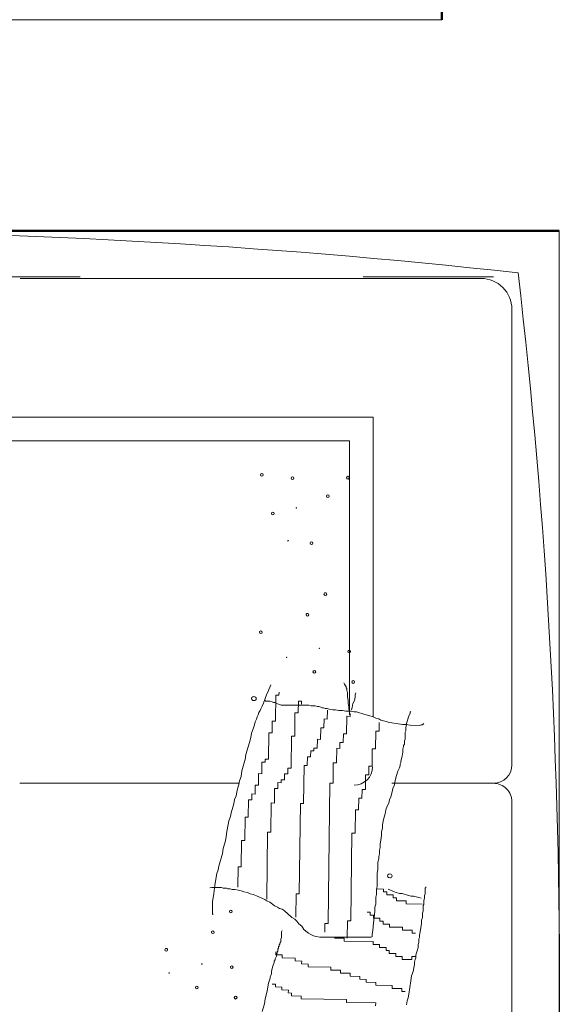
# Model space of a CAD drawing. Units: inches. Extents: x -466983 to 1020, y 324 to 318697.
# Tile 91 of 97: x 787 to 810, y 921 to 963. Entities that reach past the tile are written whole.
import ezdxf

# ---------------------------------------------------------------- set-up
doc = ezdxf.new("R2010")
doc.units = ezdxf.units.IN
doc.header["$MEASUREMENT"] = 0
for name, color, linetype, lineweight in [('A-FLOR-PATT', 252, 'Continuous', 13), ('A-FURN', 8, 'Continuous', 18), ('A-WALL', 7, 'Continuous', 50), ('L-SITE', 3, 'Continuous', 18)]:
    doc.layers.add(name, color=color, linetype=linetype, lineweight=lineweight)

# ---------------------------------------------------------------- blocks, each defined once
blk = doc.blocks.new('L Shaped Sofa')
at = {"ltscale": 2}
for p, q in [((2475.263, 723.229), (2475.263, 821.686)), ((2458.96, 739.532), (2458.96, 802.773)), ((2460.8, 737.692), (2460.8, 802.773)), ((2471.701, 760.482), (2471.701, 766.134)), ((2432.347, 748.121), (2432.347, 765.179)), ((2471.575, 729.305), (2471.575, 765.138)), ((2422.162, 750.193), (2423.138, 750.189)), ((2422.21, 750.139), (2422.162, 750.193)), ((2423.138, 750.189), (2423.772, 750.077)), ((2423.772, 750.077), (2424.406, 750.02)), ((2424.26, 750.238), (2424.213, 750.4)), ((2424.256, 749.479), (2424.26, 750.238)), ((2424.406, 750.02), (2424.747, 749.964)), ((2424.747, 749.964), (2425.332, 749.853)), ((2425.332, 749.853), (2425.624, 749.743)), ((2424.154, 748.828), (2424.155, 748.991)), ((2424.155, 748.991), (2424.205, 749.099)), ((2424.205, 749.099), (2424.206, 749.37)), ((2424.206, 749.37), (2424.256, 749.479)), ((2425.624, 749.743), (2425.916, 749.688)), ((2425.916, 749.688), (2426.89, 749.412)), ((2426.89, 749.412), (2427.28, 749.356)), ((2427.28, 749.356), (2427.865, 749.191)), ((2427.865, 749.191), (2428.206, 749.135)), ((2428.206, 749.135), (2428.596, 749.079)), ((2428.596, 749.079), (2429.132, 748.968)), ((2424.053, 748.178), (2424.103, 748.449)), ((2424.103, 748.449), (2424.104, 748.666)), ((2424.104, 748.666), (2424.154, 748.828)), ((2424.269, 748.227), (2425.857, 748.207)), ((2429.132, 748.968), (2429.425, 748.912)), ((2429.425, 748.912), (2429.766, 748.802)), ((2429.766, 748.802), (2430.058, 748.747)), ((2430.058, 748.747), (2430.74, 748.526)), ((2430.74, 748.526), (2431.081, 748.471)), ((2431.081, 748.471), (2431.373, 748.361)), ((2431.373, 748.361), (2431.666, 748.305)), ((2431.666, 748.305), (2431.909, 748.25)), ((2431.909, 748.25), (2432.25, 748.14)), ((2423.754, 747.258), (2423.853, 747.474)), ((2423.853, 747.474), (2423.904, 747.745)), ((2423.904, 747.745), (2424.003, 747.962)), ((2424.003, 747.962), (2424.053, 748.178)), ((2425.857, 748.207), (2425.853, 747.956)), ((2425.853, 747.956), (2427.895, 747.931)), ((2427.895, 747.931), (2427.892, 747.679)), ((2427.892, 747.679), (2429.707, 747.657)), ((2429.707, 747.657), (2429.704, 747.405)), ((2432.25, 748.14), (2432.543, 748.084)), ((2432.543, 748.084), (2432.884, 747.974)), ((2432.884, 747.974), (2433.322, 747.918)), ((2433.322, 747.918), (2433.858, 747.753)), ((2433.858, 747.753), (2434.199, 747.643)), ((2434.199, 747.643), (2434.589, 747.587)), ((2434.589, 747.587), (2435.174, 747.421)), ((2423.308, 746.122), (2423.605, 746.771)), ((2423.605, 746.771), (2423.704, 747.041)), ((2423.704, 747.041), (2423.754, 747.258)), ((2429.704, 747.405), (2431.065, 747.388)), ((2431.065, 747.388), (2431.061, 747.136)), ((2431.061, 747.136), (2431.515, 747.131)), ((2431.515, 747.131), (2431.512, 746.879)), ((2431.512, 746.879), (2432.193, 746.87)), ((2432.193, 746.87), (2432.19, 746.618)), ((2435.174, 747.421), (2435.515, 747.311)), ((2435.515, 747.311), (2435.904, 747.201)), ((2435.904, 747.201), (2436.246, 747.145)), ((2436.246, 747.145), (2436.586, 747.035)), ((2436.586, 747.035), (2436.879, 746.925)), ((2436.879, 746.925), (2437.122, 746.87)), ((2437.122, 746.87), (2437.317, 746.761)), ((2437.317, 746.761), (2437.512, 746.705)), ((2437.512, 746.705), (2437.658, 746.651)), ((2414.624, 746.325), (2415.208, 746.16)), ((2415.208, 746.16), (2415.598, 746.104)), ((2415.598, 746.104), (2416.183, 745.938)), ((2416.183, 745.938), (2416.524, 745.882)), ((2423.111, 745.743), (2423.21, 745.959)), ((2423.21, 745.959), (2423.308, 746.122)), ((2423.334, 745.971), (2428.551, 745.907)), ((2432.19, 746.618), (2433.097, 746.607)), ((2433.097, 746.607), (2433.094, 746.355)), ((2433.094, 746.355), (2434.001, 746.344)), ((2434.001, 746.344), (2433.998, 746.092)), ((2433.998, 746.092), (2434.225, 746.09)), ((2434.225, 746.09), (2434.222, 745.838)), ((2437.658, 746.651), (2437.852, 746.595)), ((2437.852, 746.595), (2437.998, 746.486)), ((2437.998, 746.486), (2438.144, 746.431)), ((2438.144, 746.431), (2438.339, 746.322)), ((2438.339, 746.322), (2438.582, 746.213)), ((2438.582, 746.213), (2438.923, 746.102)), ((2438.725, 745.724), (2438.727, 746.049)), ((2438.727, 746.049), (2438.777, 746.103)), ((2438.923, 746.102), (2439.215, 745.993)), ((2439.215, 745.993), (2439.556, 745.828)), ((2416.513, 744.794), (2416.519, 745.298)), ((2416.519, 745.298), (2416.746, 745.295)), ((2416.524, 745.882), (2416.816, 745.827)), ((2416.746, 745.295), (2416.749, 745.547)), ((2416.816, 745.827), (2417.06, 745.771)), ((2417.06, 745.771), (2417.206, 745.716)), ((2417.206, 745.716), (2417.304, 745.716)), ((2417.304, 745.716), (2417.401, 745.661)), ((2417.401, 745.661), (2417.547, 745.606)), ((2417.547, 745.606), (2417.742, 745.605)), ((2417.742, 745.605), (2418.132, 745.495)), ((2418.132, 745.495), (2418.424, 745.385)), ((2418.424, 745.385), (2418.522, 745.385)), ((2418.522, 745.385), (2418.619, 745.33)), ((2418.619, 745.33), (2418.716, 745.33)), ((2418.716, 745.33), (2418.911, 745.22)), ((2418.911, 745.22), (2419.057, 745.22)), ((2419.008, 744.764), (2419.015, 745.268)), ((2419.015, 745.268), (2419.241, 745.265)), ((2419.057, 745.22), (2419.155, 745.165)), ((2419.155, 745.165), (2419.252, 745.165)), ((2419.252, 745.165), (2419.301, 745.11)), ((2422.717, 745.148), (2422.816, 745.365)), ((2422.816, 745.365), (2422.963, 745.527)), ((2422.963, 745.527), (2423.111, 745.743)), ((2428.551, 745.907), (2428.548, 745.655)), ((2428.548, 745.655), (2430.816, 745.627)), ((2430.816, 745.627), (2430.813, 745.375)), ((2430.813, 745.375), (2431.947, 745.362)), ((2431.947, 745.362), (2431.944, 745.11)), ((2434.222, 745.838), (2436.263, 745.813)), ((2436.263, 745.813), (2436.26, 745.561)), ((2436.26, 745.561), (2437.168, 745.55)), ((2437.168, 745.55), (2437.165, 745.298)), ((2437.165, 745.298), (2439.206, 745.273)), ((2438.527, 745.128), (2438.626, 745.345)), ((2438.626, 745.453), (2438.676, 745.561)), ((2438.626, 745.345), (2438.626, 745.453)), ((2438.676, 745.561), (2438.725, 745.724)), ((2439.206, 745.273), (2439.203, 745.021)), ((2439.556, 745.828), (2439.994, 745.664)), ((2416.28, 744.293), (2416.286, 744.797)), ((2416.286, 744.797), (2416.513, 744.794)), ((2418.769, 743.759), (2418.782, 744.767)), ((2418.782, 744.767), (2419.008, 744.764)), ((2419.301, 745.11), (2419.447, 745.11)), ((2419.447, 745.11), (2419.544, 745.055)), ((2419.544, 745.055), (2419.642, 745.054)), ((2419.642, 745.054), (2419.69, 745)), ((2419.69, 745), (2419.788, 744.999)), ((2419.788, 744.999), (2419.836, 744.945)), ((2419.836, 744.945), (2419.934, 744.945)), ((2419.934, 744.945), (2420.031, 744.89)), ((2420.031, 744.89), (2420.226, 744.889)), ((2420.226, 744.889), (2420.372, 744.834)), ((2420.372, 744.834), (2420.812, 744.832)), ((2420.812, 744.832), (2420.909, 744.777)), ((2421.929, 744.014), (2422.469, 744.607)), ((2422.469, 744.607), (2422.568, 744.77)), ((2422.568, 744.77), (2422.618, 744.986)), ((2422.618, 744.986), (2422.717, 745.148)), ((2431.944, 745.11), (2432.398, 745.104)), ((2432.398, 745.104), (2432.395, 744.852)), ((2432.395, 744.852), (2432.622, 744.849)), ((2432.622, 744.849), (2432.619, 744.598)), ((2432.619, 744.598), (2433.072, 744.592)), ((2433.072, 744.592), (2433.069, 744.34)), ((2438.414, 742.689), (2438.427, 744.858)), ((2438.427, 744.858), (2438.477, 744.966)), ((2438.477, 744.966), (2438.527, 745.128)), ((2439.43, 745.018), (2439.203, 745.021)), ((2439.203, 745.021), (2439.43, 745.018)), ((2415.814, 743.291), (2415.823, 744.047)), ((2415.823, 744.047), (2416.05, 744.044)), ((2416.05, 744.044), (2416.053, 744.296)), ((2416.053, 744.296), (2416.28, 744.293)), ((2418.536, 743.258), (2418.542, 743.762)), ((2418.542, 743.762), (2418.769, 743.759)), ((2421.438, 743.474), (2421.634, 743.635)), ((2421.634, 743.635), (2421.781, 743.797)), ((2421.781, 743.797), (2421.929, 744.014)), ((2421.945, 743.72), (2423.76, 743.698)), ((2423.76, 743.698), (2423.757, 743.446)), ((2433.069, 744.34), (2433.523, 744.335)), ((2433.523, 744.335), (2433.52, 744.083)), ((2433.52, 744.083), (2436.015, 744.052)), ((2436.015, 744.052), (2436.012, 743.8)), ((2436.012, 743.8), (2437.827, 743.778)), ((2437.827, 743.778), (2437.823, 743.526)), ((2415.544, 739.767), (2415.587, 743.294)), ((2415.587, 743.294), (2415.814, 743.291)), ((2418.303, 742.757), (2418.309, 743.261)), ((2418.309, 743.261), (2418.536, 743.258)), ((2420.701, 742.718), (2420.849, 742.934)), ((2420.849, 742.934), (2420.996, 743.096)), ((2420.996, 743.096), (2421.241, 743.258)), ((2421.241, 743.258), (2421.438, 743.474)), ((2423.757, 743.446), (2430.788, 743.36)), ((2430.788, 743.36), (2430.785, 743.108)), ((2430.785, 743.108), (2433.734, 743.072)), ((2433.734, 743.072), (2433.731, 742.82)), ((2437.823, 743.526), (2438.731, 743.515)), ((2438.728, 743.263), (2438.501, 743.266)), ((2438.731, 743.515), (2438.728, 743.263)), ((2418.055, 740.996), (2418.076, 742.76)), ((2418.076, 742.76), (2418.303, 742.757)), ((2420.403, 741.852), (2420.453, 742.123)), ((2420.453, 742.123), (2420.504, 742.339)), ((2420.504, 742.339), (2420.603, 742.556)), ((2420.603, 742.556), (2420.701, 742.718)), ((2433.731, 742.82), (2434.412, 742.812)), ((2434.412, 742.812), (2434.409, 742.56)), ((2434.409, 742.56), (2434.862, 742.555)), ((2434.862, 742.555), (2434.859, 742.303)), ((2434.859, 742.303), (2435.086, 742.3)), ((2435.086, 742.3), (2435.083, 742.048)), ((2438.312, 742.039), (2438.362, 742.201)), ((2438.362, 742.201), (2438.364, 742.527)), ((2438.364, 742.527), (2438.414, 742.689)), ((2420.378, 737.84), (2420.403, 741.852)), ((2420.783, 741.467), (2421.464, 741.459)), ((2421.464, 741.459), (2421.46, 741.207)), ((2435.083, 742.048), (2435.764, 742.04)), ((2435.764, 742.04), (2435.76, 741.788)), ((2435.76, 741.788), (2436.668, 741.777)), ((2436.668, 741.777), (2436.665, 741.525)), ((2436.665, 741.525), (2437.345, 741.516)), ((2437.345, 741.516), (2437.342, 741.265)), ((2438.161, 741.281), (2438.162, 741.443)), ((2438.162, 741.443), (2438.212, 741.552)), ((2438.212, 741.552), (2438.213, 741.66)), ((2438.213, 741.66), (2438.262, 741.768)), ((2438.262, 741.768), (2438.312, 741.931)), ((2438.312, 741.931), (2438.312, 742.039)), ((2417.819, 740.243), (2417.828, 740.999)), ((2417.828, 740.999), (2418.055, 740.996)), ((2420.311, 739.961), (2420.32, 740.717)), ((2421.46, 741.207), (2432.349, 741.074)), ((2432.349, 741.074), (2432.346, 740.822)), ((2432.346, 740.822), (2433.933, 740.802)), ((2433.933, 740.802), (2433.93, 740.55)), ((2437.342, 741.265), (2438.023, 741.256)), ((2438.009, 740.36), (2438.06, 740.631)), ((2438.06, 740.631), (2438.061, 740.847)), ((2438.061, 740.847), (2438.112, 741.118)), ((2438.112, 741.118), (2438.161, 741.281)), ((2417.583, 739.49), (2417.592, 740.246)), ((2417.592, 740.246), (2417.819, 740.243)), ((2420.056, 737.696), (2420.084, 739.964)), ((2420.084, 739.964), (2420.311, 739.961)), ((2433.93, 740.55), (2435.065, 740.536)), ((2435.065, 740.536), (2435.061, 740.285)), ((2435.061, 740.285), (2435.515, 740.279)), ((2435.515, 740.279), (2435.512, 740.027)), ((2435.512, 740.027), (2436.193, 740.019)), ((2436.193, 740.019), (2436.189, 739.767)), ((2437.955, 739.384), (2437.957, 739.818)), ((2437.957, 739.818), (2438.008, 740.089)), ((2438.008, 740.089), (2438.009, 740.36)), ((2439.714, 739.755), (2439.763, 739.809)), ((2439.763, 739.809), (2439.86, 739.809)), ((2439.86, 739.809), (2439.909, 739.863)), ((2439.909, 739.863), (2440.056, 739.916)), ((2440.056, 739.916), (2440.154, 739.97)), ((2415.29, 737.503), (2415.317, 739.77)), ((2415.317, 739.77), (2415.544, 739.767)), ((2417.347, 738.737), (2417.356, 739.493)), ((2417.356, 739.493), (2417.583, 739.49)), ((2420.308, 739.709), (2421.669, 739.692)), ((2421.669, 739.692), (2421.666, 739.44)), ((2421.666, 739.44), (2428.471, 739.357)), ((2428.471, 739.357), (2428.468, 739.105)), ((2428.468, 739.105), (2430.282, 739.083)), ((2430.282, 739.083), (2430.279, 738.831)), ((2436.189, 739.767), (2437.55, 739.75)), ((2437.55, 739.75), (2437.547, 739.498)), ((2437.547, 739.498), (2437.774, 739.496)), ((2437.663, 739.548), (2437.907, 739.547)), ((2437.904, 739.005), (2437.905, 739.167)), ((2437.905, 739.167), (2437.955, 739.384)), ((2437.907, 739.547), (2438.102, 739.6)), ((2458.96, 739.532), (2437.956, 739.532)), ((2438.052, 739.384), (2438.247, 739.328)), ((2438.102, 739.6), (2438.298, 739.599)), ((2438.247, 739.328), (2438.54, 739.273)), ((2438.298, 739.599), (2438.542, 739.652)), ((2438.54, 739.273), (2438.783, 739.163)), ((2438.542, 739.652), (2438.786, 739.651)), ((2438.783, 739.163), (2439.026, 739.108)), ((2438.786, 739.651), (2439.03, 739.704)), ((2439.026, 739.108), (2439.222, 739.107)), ((2439.03, 739.704), (2439.42, 739.702)), ((2439.222, 739.107), (2439.368, 739.052)), ((2439.42, 739.702), (2439.518, 739.756)), ((2439.518, 739.756), (2439.714, 739.755)), ((2417.114, 738.236), (2417.12, 738.74)), ((2417.12, 738.74), (2417.347, 738.737)), ((2430.279, 738.831), (2431.187, 738.82)), ((2431.187, 738.82), (2431.184, 738.568)), ((2431.184, 738.568), (2431.864, 738.56)), ((2431.864, 738.56), (2431.861, 738.308)), ((2431.861, 738.308), (2432.995, 738.294)), ((2432.995, 738.294), (2432.992, 738.042)), ((2437.655, 738.247), (2437.704, 738.355)), ((2437.704, 738.355), (2437.904, 739.005)), ((2471.701, 738.472), (2471.701, 736.259)), ((2416.878, 737.483), (2416.887, 738.239)), ((2416.887, 738.239), (2417.114, 738.236)), ((2419.823, 737.195), (2419.83, 737.699)), ((2419.83, 737.699), (2420.056, 737.696)), ((2420.427, 737.786), (2420.622, 737.785)), ((2420.622, 737.785), (2420.915, 737.729)), ((2420.915, 737.729), (2421.5, 737.672)), ((2421.5, 737.672), (2421.89, 737.616)), ((2421.865, 737.17), (2421.871, 737.674)), ((2421.871, 737.674), (2422.098, 737.672)), ((2421.89, 737.616), (2422.426, 737.559)), ((2422.098, 737.672), (2422.101, 737.923)), ((2422.101, 737.923), (2422.328, 737.921)), ((2422.328, 737.921), (2422.331, 738.173)), ((2422.426, 737.559), (2422.719, 737.558)), ((2422.719, 737.558), (2422.963, 737.503)), ((2432.992, 738.042), (2433.673, 738.034)), ((2433.673, 738.034), (2433.67, 737.782)), ((2433.67, 737.782), (2435.031, 737.765)), ((2435.031, 737.765), (2435.028, 737.514)), ((2435.028, 737.514), (2436.389, 737.497)), ((2437.406, 737.489), (2437.505, 737.705)), ((2460.8, 737.692), (2437.499, 737.692)), ((2437.505, 737.705), (2437.605, 738.03)), ((2437.605, 738.03), (2437.655, 738.247)), ((2415.063, 737.506), (2415.29, 737.503)), ((2416.635, 736.227), (2416.651, 737.486)), ((2416.651, 737.486), (2416.878, 737.483)), ((2419.59, 736.694), (2419.597, 737.198)), ((2419.597, 737.198), (2419.823, 737.195)), ((2421.402, 736.42), (2421.408, 736.924)), ((2421.408, 736.924), (2421.635, 736.921)), ((2421.635, 736.921), (2421.638, 737.173)), ((2421.638, 737.173), (2421.865, 737.17)), ((2422.963, 737.503), (2423.499, 737.5)), ((2423.499, 737.5), (2423.694, 737.445)), ((2423.694, 737.445), (2424.133, 737.443)), ((2423.9, 736.642), (2423.903, 736.894)), ((2423.903, 736.894), (2424.13, 736.891)), ((2424.13, 736.891), (2424.136, 737.395)), ((2424.133, 737.443), (2424.328, 737.388)), ((2424.328, 737.388), (2425.353, 737.383)), ((2425.353, 737.383), (2425.645, 737.327)), ((2425.645, 737.327), (2426.231, 737.325)), ((2426.231, 737.325), (2426.475, 737.269)), ((2426.475, 737.269), (2426.67, 737.268)), ((2426.67, 737.268), (2426.865, 737.213)), ((2426.865, 737.213), (2427.157, 737.212)), ((2427.157, 737.212), (2427.352, 737.157)), ((2427.352, 737.157), (2427.645, 737.155)), ((2427.645, 737.155), (2427.937, 737.1)), ((2427.937, 737.1), (2428.279, 737.044)), ((2428.279, 737.044), (2428.571, 737.043)), ((2428.571, 737.043), (2428.864, 736.987)), ((2428.864, 736.987), (2429.108, 736.986)), ((2429.108, 736.986), (2429.4, 736.93)), ((2429.4, 736.93), (2429.644, 736.875)), ((2429.644, 736.875), (2429.985, 736.765)), ((2429.985, 736.765), (2430.277, 736.709)), ((2436.389, 737.497), (2436.386, 737.245)), ((2436.386, 737.245), (2437.066, 737.237)), ((2437.157, 736.677), (2437.258, 737.11)), ((2437.258, 737.11), (2437.356, 737.272)), ((2437.356, 737.272), (2437.406, 737.489)), ((2416.399, 735.474), (2416.409, 736.229)), ((2416.409, 736.229), (2416.635, 736.227)), ((2419.127, 735.944), (2419.134, 736.448)), ((2419.134, 736.448), (2419.36, 736.445)), ((2419.36, 736.445), (2419.364, 736.697)), ((2419.364, 736.697), (2419.59, 736.694)), ((2421.163, 735.415), (2421.175, 736.423)), ((2421.175, 736.423), (2421.402, 736.42)), ((2423.437, 735.892), (2423.44, 736.143)), ((2423.44, 736.143), (2423.667, 736.141)), ((2423.667, 736.141), (2423.673, 736.644)), ((2423.673, 736.644), (2423.9, 736.642)), ((2423.88, 735.98), (2424.128, 736.521)), ((2430.277, 736.709), (2430.569, 736.599)), ((2430.569, 736.599), (2430.813, 736.49)), ((2430.813, 736.49), (2431.056, 736.434)), ((2431.056, 736.434), (2431.3, 736.325)), ((2431.3, 736.325), (2431.689, 736.215)), ((2431.689, 736.215), (2431.933, 736.159)), ((2431.933, 736.159), (2432.225, 736.049)), ((2432.225, 736.049), (2432.566, 735.994)), ((2432.347, 728.35), (2432.347, 736.259)), ((2432.566, 735.994), (2432.956, 735.883)), ((2436.906, 735.431), (2437.057, 736.244)), ((2437.057, 736.244), (2437.058, 736.461)), ((2437.058, 736.461), (2437.157, 736.677)), ((2471.701, 728.35), (2471.701, 736.259)), ((2416.169, 735.224), (2416.172, 735.476)), ((2416.172, 735.476), (2416.399, 735.474)), ((2418.658, 734.69), (2418.668, 735.446)), ((2418.668, 735.446), (2418.895, 735.443)), ((2418.895, 735.443), (2418.901, 735.947)), ((2418.901, 735.947), (2419.127, 735.944)), ((2420.927, 734.662), (2420.936, 735.418)), ((2420.936, 735.418), (2421.163, 735.415)), ((2423.201, 735.139), (2423.211, 735.894)), ((2423.211, 735.894), (2423.437, 735.892)), ((2423.63, 734.951), (2423.78, 735.439)), ((2423.78, 735.439), (2423.781, 735.655)), ((2423.781, 735.655), (2423.88, 735.98)), ((2432.956, 735.883), (2433.297, 735.773)), ((2433.297, 735.773), (2433.54, 735.664)), ((2433.54, 735.664), (2433.735, 735.609)), ((2433.735, 735.609), (2433.833, 735.608)), ((2433.833, 735.608), (2433.93, 735.554)), ((2433.93, 735.554), (2434.076, 735.553)), ((2434.076, 735.553), (2434.466, 735.443)), ((2434.466, 735.443), (2434.758, 735.387)), ((2434.758, 735.387), (2435.002, 735.386)), ((2435.002, 735.386), (2435.197, 735.331)), ((2435.197, 735.331), (2435.295, 735.33)), ((2435.295, 735.33), (2435.392, 735.276)), ((2435.392, 735.276), (2435.636, 735.274)), ((2435.636, 735.274), (2435.782, 735.22)), ((2435.782, 735.22), (2436.319, 735.217)), ((2436.319, 735.217), (2436.416, 735.162)), ((2436.904, 735.16), (2436.906, 735.431)), ((2415.14, 735.1), (2415.433, 735.044)), ((2415.433, 735.044), (2415.677, 734.989)), ((2415.677, 734.989), (2415.969, 734.933)), ((2415.969, 734.933), (2416.993, 734.766)), ((2416.993, 734.766), (2417.383, 734.709)), ((2417.383, 734.709), (2417.724, 734.599)), ((2417.724, 734.599), (2418.016, 734.544)), ((2418.016, 734.544), (2418.26, 734.488)), ((2418.26, 734.488), (2418.455, 734.488)), ((2418.455, 734.488), (2418.65, 734.432)), ((2418.885, 734.687), (2418.658, 734.69)), ((2418.882, 734.435), (2418.885, 734.687)), ((2420.697, 734.413), (2420.7, 734.665)), ((2420.7, 734.665), (2420.927, 734.662)), ((2422.959, 733.882), (2422.974, 735.141)), ((2422.974, 735.141), (2423.201, 735.139)), ((2423.479, 734.139), (2423.579, 734.572)), ((2423.579, 734.572), (2423.58, 734.735)), ((2423.58, 734.735), (2423.63, 734.951)), ((2436.416, 735.162), (2436.709, 735.161)), ((2436.709, 735.161), (2436.855, 735.106)), ((2436.849, 734.076), (2436.853, 734.835)), ((2436.853, 734.835), (2436.904, 735.16)), ((2436.855, 735.106), (2437.001, 735.105)), ((2437.001, 735.105), (2437.586, 734.94)), ((2437.586, 734.94), (2437.78, 734.831)), ((2437.78, 734.831), (2437.878, 734.83)), ((2437.878, 734.83), (2437.926, 734.776)), ((2418.65, 734.432), (2418.796, 734.378)), ((2418.796, 734.378), (2418.991, 734.377)), ((2418.991, 734.377), (2419.186, 734.321)), ((2419.186, 734.321), (2419.332, 734.267)), ((2419.332, 734.267), (2419.575, 734.211)), ((2419.575, 734.211), (2419.819, 734.21)), ((2419.819, 734.21), (2419.966, 734.155)), ((2419.966, 734.155), (2420.258, 734.154)), ((2420.258, 734.154), (2420.356, 734.099)), ((2420.356, 734.099), (2420.551, 734.098)), ((2420.551, 734.098), (2420.794, 734.043)), ((2420.794, 734.043), (2421.136, 733.987)), ((2421.136, 733.987), (2421.428, 733.931)), ((2421.428, 733.931), (2421.721, 733.93)), ((2421.721, 733.93), (2421.916, 733.875)), ((2421.916, 733.875), (2422.257, 733.873)), ((2422.257, 733.873), (2422.403, 733.818)), ((2422.403, 733.818), (2422.842, 733.816)), ((2422.842, 733.816), (2422.94, 733.762)), ((2422.94, 733.762), (2423.232, 733.76)), ((2423.232, 733.76), (2423.427, 733.705)), ((2423.427, 733.705), (2423.622, 733.704)), ((2423.429, 733.976), (2423.479, 734.139)), ((2423.622, 733.704), (2423.769, 733.649)), ((2436.897, 733.967), (2436.849, 734.076)), ((2436.896, 733.859), (2436.897, 733.967)), ((2436.993, 733.75), (2436.896, 733.859)), ((2423.769, 733.649), (2424.208, 733.647)), ((2424.208, 733.647), (2424.256, 733.593)), ((2424.256, 733.593), (2424.305, 733.593)), ((2430.914, 726.917), (2396.145, 726.917)), ((2469.187, 726.917), (2433.78, 726.917)), ((2475.263, 723.229), (2377.232, 723.229))]:
    blk.add_line(p, q, dxfattribs=at)
for centre, radius, start, end in [((1939.075, 785.436), 536.188, 353.68225, 6.54157), ((2417.604, 753.562), 0.0177, 90, 270), ((2417.604, 753.562), 0.0177, 270, 90), ((2419.413, 753.788), 0.106, 90, 270), ((2419.413, 753.788), 0.106, 270, 90), ((2416.474, 751.412), 0.106, 90, 270), ((2416.474, 751.412), 0.106, 270, 90), ((2418.303, 751.018), 0.0177, 90, 270), ((2418.303, 751.018), 0.0177, 270, 90), ((2420.77, 750.168), 0.106, 90, 270), ((2420.77, 750.168), 0.106, 270, 90), ((2415.692, 748.389), 0.106, 90, 270), ((2415.692, 748.389), 0.106, 270, 90), ((2418.057, 748.697), 0.106, 90, 270), ((2418.057, 748.697), 0.106, 270, 90), ((2422.376, 748.771), 0.106, 90, 270), ((2422.376, 748.771), 0.106, 270, 90), ((2444.081, 746.436), 0.106, 90, 270), ((2444.081, 746.436), 0.106, 270, 90), ((2456.312, 746.349), 0.106, 1.3946, 181.3946), ((2456.312, 746.349), 0.106, 181.3946, 1.3946), ((2453.309, 745.494), 0.106, 1.3946, 181.3946), ((2453.309, 745.494), 0.106, 181.3946, 1.3946), ((2442.129, 744.423), 0.0177, 90, 270), ((2442.129, 744.423), 0.0177, 270, 90), ((2451.187, 744.312), 0.0177, 1.3946, 181.3946), ((2451.187, 744.312), 0.0177, 181.3946, 1.3946), ((2453.747, 743.675), 0.0177, 1.3946, 181.3946), ((2453.747, 743.675), 0.0177, 181.3946, 1.3946), ((2456.062, 743.978), 0.106, 1.3946, 181.3946), ((2456.062, 743.978), 0.106, 181.3946, 1.3946), ((2445.438, 742.815), 0.106, 90, 270), ((2445.438, 742.815), 0.106, 270, 90), ((2440.998, 742.273), 0.106, 90, 270), ((2440.998, 742.273), 0.106, 270, 90), ((2451.005, 742.498), 0.106, 1.3946, 181.3946), ((2451.005, 742.498), 0.106, 181.3946, 1.3946), ((2442.827, 741.879), 0.0177, 90, 270), ((2442.827, 741.879), 0.0177, 270, 90), ((2447.044, 741.419), 0.106, 90, 270), ((2447.044, 741.419), 0.106, 270, 90), ((2454.657, 741.23), 0.106, 1.3946, 181.3946), ((2454.657, 741.23), 0.106, 181.3946, 1.3946), ((2433.636, 739.178), 1.433, 180, 270), ((2440.217, 739.25), 0.106, 90, 270), ((2440.217, 739.25), 0.106, 270, 90), ((2442.581, 739.558), 0.106, 90, 270), ((2442.581, 739.558), 0.106, 270, 90), ((2456.093, 739.658), 0.106, 1.3946, 181.3946), ((2456.093, 739.658), 0.106, 181.3946, 1.3946), ((2469.187, 729.305), 2.388, 270, 0), ((2430.914, 728.35), 1.433, 270, 0), ((2433.78, 728.35), 1.433, 180, 270), ((2416.36, 1205.029), 481.82, 262.88673, 276.63201)]:
    blk.add_arc(centre, radius, start, end, dxfattribs=at)
at = {"ltscale": 2, "extrusion": (0, 0, -1)}
for centre, start_param, end_param in [((2438.928, 746.97), -1.570796, 1.570796), ((2438.928, 746.97), 1.570796, 4.712389), ((2425.152, 736.408), -1.570796, 1.570796), ((2425.152, 736.408), 1.570796, 4.712389)]:
    blk.add_ellipse(centre, major_axis=(-0.002, -0.177), ratio=0.9, start_param=start_param, end_param=end_param, dxfattribs=at)

msp = doc.modelspace()

# ---------------------------------------------------------------- hatches: boundary and pattern name
at = {"layer": 'A-FLOR-PATT', "transparency": 33554572}
h = msp.add_hatch(dxfattribs=at)
h.set_pattern_fill('ANSI37', color=256, scale=30)
h.set_pattern_definition([(45, (-1212.4137, -290.035), (-2.6516504, 2.6516504), []), (135, (-1212.4137, -290.035), (-2.6516504, -2.6516504), [])])
h.paths.add_polyline_path([(901.806, 1075.938), (900.614, 1075.938), (900.614, 1065.386), (899.391, 1065.386), (898.091, 1065.386), (892.836, 1058.71, -0.258377), (892.188, 1058.351), (879.985, 1058.351, -0.20177), (879.438, 1058.581), (874.081, 1065.386), (872.781, 1065.386), (871.558, 1065.386), (871.558, 1075.938), (813.806, 1075.938), (813.806, 1044.792), (832.395, 1044.792, -0.394795), (848.66, 1028.536), (848.66, 1009.938), (901.806, 1009.938), (901.806, 1015.938), (901.306, 1015.938), (871.306, 1015.938), (871.306, 1017.25), (871.334, 1017.25, -0.401453), (901.306, 1045.938), (901.806, 1045.938)])
edge = h.paths.add_edge_path(flags=16)
edge.add_line((847.773, 1068.949), (847.773, 1073.709))
edge.add_arc((849.227, 1073.709), 1.454, 90, 180, ccw=False)
edge.add_line((849.227, 1075.163), (864.492, 1075.163))
edge.add_arc((864.492, 1073.709), 1.454, 0, 90, ccw=False)
edge.add_line((865.946, 1073.709), (865.946, 1069.004))
edge.add_arc((832.645, 1068.976), 33.301, -20.6123, 0.0472, ccw=False)
edge.add_ellipse((856.859, 1058.48), major_axis=(0, 10.213), ratio=0.685919, start_angle=100.0088, end_angle=259.9912, ccw=False)
edge.add_arc((881.074, 1068.976), 33.301, 180.0472, 200.6123, ccw=False)
h.paths.add_polyline_path([(853.146, 1066.482), (853.146, 1066.453), (853.146, 1066.453, 0.433107), (852.917, 1066.685), (852.917, 1066.453), (853.146, 1066.453), (853.146, 1066.482), (853.088, 1066.612, 0.697939), (852.7, 1066.453), (852.7, 1066.453), (852.7, 1066.482), (852.917, 1067.001), (852.917, 1066.685, -0.396254)], flags=0)
h.paths.add_polyline_path([(861.019, 1066.482), (861.019, 1066.453), (861.019, 1066.453, 0.416404), (860.802, 1066.685), (860.802, 1066.453), (861.019, 1066.453), (861.019, 1066.482), (860.967, 1066.605, 0.713344), (860.573, 1066.453), (860.573, 1066.453), (860.573, 1066.482), (860.802, 1067.001), (860.802, 1066.685, -0.379973)], flags=0)
edge = h.paths.add_edge_path(flags=0)
edge.add_spline(control_points=[(861.13, 1065.785), (861.466, 1065.248), (861.613, 1065.016), (861.983, 1064.374), (862.192, 1063.944), (862.561, 1063.039), (862.721, 1062.563), (862.987, 1061.578), (863.092, 1061.069), (863.245, 1060.031), (863.293, 1059.503), (863.329, 1058.441), (863.318, 1057.908), (863.237, 1056.852), (863.166, 1056.329), (862.97, 1055.308), (862.843, 1054.81), (862.537, 1053.852), (862.357, 1053.393), (861.951, 1052.525), (861.725, 1052.117), (861.233, 1051.362), (860.967, 1051.016), (860.405, 1050.395), (860.108, 1050.12), (859.494, 1049.646), (859.176, 1049.448), (858.528, 1049.13), (858.197, 1049.011), (857.531, 1048.852), (857.196, 1048.812), (856.525, 1048.812), (856.189, 1048.852), (855.524, 1049.01), (855.193, 1049.129), (854.545, 1049.447), (854.227, 1049.645), (853.612, 1050.118), (853.316, 1050.393), (852.753, 1051.014), (852.487, 1051.36), (851.995, 1052.114), (851.769, 1052.523), (851.363, 1053.39), (851.183, 1053.85), (850.877, 1054.807), (850.75, 1055.305), (850.553, 1056.326), (850.483, 1056.849), (850.401, 1057.905), (850.39, 1058.438), (850.426, 1059.5), (850.473, 1060.028), (850.626, 1061.066), (850.732, 1061.575), (850.997, 1062.561), (851.157, 1063.036), (851.525, 1063.942), (851.734, 1064.371), (852.106, 1065.016), (852.254, 1065.25), (852.608, 1065.733)], knot_values=[3.915332, 3.915332, 3.915332, 3.915332, 4.013468, 4.013468, 4.175532, 4.175532, 4.337596, 4.337596, 4.49966, 4.49966, 4.661724, 4.661724, 4.823788, 4.823788, 4.985852, 4.985852, 5.147916, 5.147916, 5.30998, 5.30998, 5.472044, 5.472044, 5.634109, 5.634109, 5.796173, 5.796173, 5.958237, 5.958237, 6.120301, 6.120301, 6.282365, 6.282365, 6.444429, 6.444429, 6.606493, 6.606493, 6.768557, 6.768557, 6.930621, 6.930621, 7.092685, 7.092685, 7.254749, 7.254749, 7.416813, 7.416813, 7.578878, 7.578878, 7.740942, 7.740942, 7.903006, 7.903006, 8.06507, 8.06507, 8.227134, 8.227134, 8.389198, 8.389198, 8.551262, 8.551262, 8.65037, 8.65037, 8.65037, 8.65037], degree=3, periodic=0)
edge.add_line((852.642, 1065.785), (861.13, 1065.785))
edge = h.paths.add_edge_path(flags=0)
edge.add_ellipse((856.85, 1057.743), major_axis=(0, 7.792), ratio=0.687861, start_angle=0, end_angle=360)
h.paths.add_polyline_path([(848.863, 1069.389), (848.863, 1073.96, -0.414214), (849.954, 1075.051), (863.765, 1075.051, -0.414214), (864.856, 1073.96), (864.856, 1069.389, -0.388936), (864.524, 1069.027, -0.043561), (849.195, 1069.027, -0.388936)], flags=0)
h.paths.add_polyline_path([(853.101, 1068.112, -1), (852.677, 1068.112, -1)], flags=0)
edge = h.paths.add_edge_path(flags=0)
edge.add_ellipse((856.859, 1057.338), major_axis=(0, 2.207), ratio=0.657164, start_angle=0, end_angle=360)
h.paths.add_polyline_path([(861.041, 1068.112, -1), (860.618, 1068.112, -1)], flags=0)
edge = h.paths.add_edge_path()
edge.add_line((573.954, 1057.341), (573.954, 1075.938))
edge.add_line((573.954, 1075.938), (558.731, 1075.938))
edge.add_line((558.731, 1075.938), (558.731, 1065.386))
edge.add_line((558.731, 1065.386), (557.507, 1065.386))
edge.add_line((557.507, 1065.386), (556.207, 1065.386))
edge.add_line((556.207, 1065.386), (550.952, 1058.71))
edge.add_arc((550.304, 1059.116), 0.765, 270, 327.9483, ccw=False)
edge.add_line((550.304, 1058.351), (538.101, 1058.351))
edge.add_arc((538.101, 1059.116), 0.765, 224.3704, 270, ccw=False)
edge.add_line((537.555, 1058.581), (532.198, 1065.386))
edge.add_line((532.198, 1065.386), (530.898, 1065.386))
edge.add_line((530.898, 1065.386), (529.674, 1065.386))
edge.add_line((529.674, 1065.386), (529.674, 1075.938))
edge.add_line((529.674, 1075.938), (520.806, 1075.938))
edge.add_line((520.806, 1075.938), (520.806, 1045.938))
edge.add_line((520.806, 1045.938), (521.306, 1045.938))
edge.add_arc((521.306, 1015.938), 30, 2.5075, 90, ccw=False)
edge.add_line((551.277, 1017.25), (551.306, 1017.25))
edge.add_line((551.306, 1017.25), (551.306, 1015.938))
edge.add_line((551.306, 1015.938), (520.806, 1015.938))
edge.add_line((520.806, 1015.938), (520.806, 1009.938))
edge.add_line((520.806, 1009.938), (559.191, 1010.402))
edge.add_arc((559.191, 1011.856), 1.454, 180, 270, ccw=False)
edge.add_line((557.737, 1011.856), (557.737, 1016.561))
edge.add_arc((591.039, 1016.589), 33.301, 159.3877, 180.0472, ccw=False)
edge.add_ellipse((566.824, 1027.085), major_axis=(0, 10.213), ratio=0.685919, start_angle=280.0088, end_angle=439.9912, ccw=False)
edge.add_arc((542.609, 1016.589), 33.301, 0.0472, 20.6123, ccw=False)
edge.add_line((575.91, 1016.616), (575.91, 1011.856))
edge.add_arc((574.456, 1011.856), 1.454, -90, 0, ccw=False)
edge.add_line((574.456, 1010.402), (608.806, 1009.938))
edge.add_line((608.806, 1009.938), (608.806, 1041.086))
edge.add_line((608.806, 1041.086), (590.218, 1041.086))
edge.add_arc((590.775, 1057.907), 16.831, 181.9277, 268.1032, ccw=False)
edge = h.paths.add_edge_path()
edge.add_ellipse((494.244, 583.62), major_axis=(0, 10.213), ratio=0.685919, start_angle=280.0088, end_angle=439.9912, ccw=False)
edge.add_arc((470.03, 573.124), 33.301, 0.0472, 20.6123, ccw=False)
edge.add_line((503.331, 573.152), (503.331, 568.392))
edge.add_arc((501.877, 568.392), 1.454, -90, 0, ccw=False)
edge.add_line((501.877, 566.938), (539.806, 566.938))
edge.add_line((539.806, 566.938), (539.806, 572.938))
edge.add_line((539.806, 572.938), (539.306, 572.938))
edge.add_line((539.306, 572.938), (509.306, 572.938))
edge.add_line((509.306, 572.938), (509.306, 574.25))
edge.add_line((509.306, 574.25), (509.334, 574.25))
edge.add_arc((539.306, 572.938), 30, 90, 177.4925, ccw=False)
edge.add_line((539.306, 602.938), (539.806, 602.938))
edge.add_line((539.806, 602.938), (539.806, 626.938))
edge.add_line((539.806, 626.938), (531.772, 626.938))
edge.add_line((531.772, 626.938), (531.772, 616.386))
edge.add_line((531.772, 616.386), (530.548, 616.386))
edge.add_line((530.548, 616.386), (529.249, 616.386))
edge.add_line((529.249, 616.386), (523.711, 609.351))
edge.add_line((523.711, 609.351), (510.777, 609.351))
edge.add_line((510.777, 609.351), (505.239, 616.386))
edge.add_line((505.239, 616.386), (503.939, 616.386))
edge.add_line((503.939, 616.386), (502.715, 616.386))
edge.add_line((502.715, 616.386), (502.715, 626.938))
edge.add_line((502.715, 626.938), (481.698, 626.938))
edge.add_line((481.698, 626.938), (481.698, 610.995))
edge.add_arc((467.27, 611.473), 14.436, 271.9277, 358.1032, ccw=False)
edge.add_line((467.756, 597.045), (451.806, 597.045))
edge.add_line((451.806, 597.045), (451.806, 584.404))
edge.add_line((451.806, 584.404), (451.806, 566.938))
edge.add_line((451.806, 566.938), (486.612, 566.938))
edge.add_arc((486.612, 568.392), 1.454, 180, 270, ccw=False)
edge.add_line((485.158, 568.392), (485.158, 573.097))
edge.add_arc((518.459, 573.124), 33.301, 159.3877, 180.0472, ccw=False)
h.paths.add_polyline_path([(836.261, 1020.733), (879.89, 1020.733), (879.89, 1039.39), (836.261, 1039.39)], flags=25)
h.paths.add_polyline_path([(549.985, 1036.749), (593.614, 1036.749), (593.614, 1055.407), (549.985, 1055.407)], flags=24)
h.paths.add_polyline_path([(475.123, 595.596), (518.752, 595.596), (518.752, 614.253), (475.123, 614.253)], flags=24)
h = msp.add_hatch(dxfattribs=at)
h.set_pattern_fill('ANSI37', color=256, scale=20)
h.set_pattern_definition([(45, (-1212.4137, -290.035), (-1.767767, 1.767767), []), (135, (-1212.4137, -290.035), (-1.767767, -1.767767), [])])
h.paths.add_polyline_path([(809.806, 870.938), (809.806, 888.152), (806.998, 888.152), (802.662, 888.152), (789.383, 888.152), (786.285, 888.152, -0.414214), (785.499, 888.937), (785.499, 900.196), (785.499, 908.47, -0.414214), (786.808, 909.779, -0.414214), (785.499, 911.088), (785.499, 929.101, -0.414214), (786.808, 930.411, -0.414214), (785.499, 931.72), (785.499, 931.904, -0.414214), (784.19, 930.595), (766.722, 930.595, -0.412359), (765.413, 931.896, -0.413741), (764.115, 930.578), (744.578, 930.422, -0.416556), (743.786, 931.207), (743.786, 933.515), (742.215, 933.515), (742.215, 952.024, -0.001344), (743.786, 952.2), (743.786, 953.938), (678.592, 953.938), (678.592, 951.131), (678.592, 946.794), (678.592, 933.515), (678.592, 930.417, -0.414214), (677.806, 929.631), (666.548, 929.631), (658.274, 929.631, -0.414214), (656.965, 930.94, -0.414214), (655.656, 929.631), (637.642, 929.631, -0.414214), (636.333, 930.94, -0.414214), (635.024, 929.631), (634.839, 929.631, -0.414214), (636.149, 928.322), (636.149, 910.854, -0.412359), (634.848, 909.545, -0.413741), (636.165, 908.247), (636.321, 888.71, -0.416556), (635.536, 887.918), (633.228, 887.918), (633.228, 886.347), (614.719, 886.347, -0.001344), (614.544, 887.918), (612.806, 887.918), (612.806, 834.938), (612.806, 752.938), (612.806, 748.938), (612.806, 697.938), (654.806, 697.938), (654.806, 701.938), (715.806, 701.938), (715.806, 737.435), (774.292, 737.435), (774.292, 795.938), (809.806, 795.938)])
h.paths.add_polyline_path([(679.276, 849.576, 0.102523), (682.148, 849.261, -0.080461), (694.543, 849.773, -0.283899), (694.482, 849.008, 0.136605), (694.407, 848.81, -0.030441), (694.543, 846.893), (694.543, 842.62), (694.543, 838.347, -0.028219), (694.425, 836.568), (694.425, 836.568, 0.196187), (694.446, 836.271, -0.302897), (694.543, 835.467, -0.080461), (682.148, 835.979, 0.102523), (679.276, 835.664, -0.58611), (678.646, 836.017), (678.646, 849.223, -0.58611)], flags=16)
h.paths.add_polyline_path([(679.517, 848.651, 0.699597), (679.476, 848.634, 1.20716), (679.194, 848.742, 0.010621)], flags=0)
h.paths.add_polyline_path([(679.492, 836.561, -0.013798), (679.918, 836.659, -0.071703), (682.853, 837.143, -0.165743), (682.166, 839.101), (682.166, 842.609), (682.166, 846.06, -0.240616), (683.473, 848.677, -0.068263), (693.929, 849.008), (693.788, 848.708), (693.788, 849.023, 0.067332), (683.473, 848.677, 0.240616), (682.166, 846.06), (682.166, 842.609), (682.166, 839.101, 0.23459), (683.461, 836.551, 0.068093), (693.788, 836.195), (693.788, 836.51), (693.93, 836.21, -0.077215), (682.242, 836.782, 0.086627), (679.528, 836.57, -0.628402), (679.503, 836.573), (679.503, 836.607, 0.910458)], flags=0)
h.paths.add_polyline_path([(679.476, 848.636), (679.207, 848.647), (679.207, 836.572, 0.913566), (679.365, 836.586), (679.476, 836.582)], flags=0)
h.paths.add_polyline_path([(679.276, 829.86, 0.102523), (682.148, 829.546, -0.080461), (694.543, 830.057, -0.283899), (694.482, 829.293, 0.136605), (694.407, 829.095, -0.030441), (694.543, 827.178), (694.543, 822.904), (694.543, 818.631, -0.028219), (694.425, 816.853), (694.425, 816.853, 0.196187), (694.446, 816.556, -0.302897), (694.543, 815.752, -0.080461), (682.148, 816.263, 0.102523), (679.276, 815.949, -0.58611), (678.646, 816.302), (678.646, 829.507, -0.58611)], flags=16)
h.paths.add_polyline_path([(679.517, 828.936, 0.699597), (679.476, 828.919, 1.20716), (679.194, 829.027, 0.010621)], flags=0)
h.paths.add_polyline_path([(679.492, 816.846, -0.013798), (679.918, 816.944, -0.071703), (682.853, 817.428, -0.165743), (682.166, 819.385), (682.166, 822.894), (682.166, 826.345, -0.240616), (683.473, 828.961, -0.068263), (693.929, 829.293), (693.788, 828.993), (693.788, 829.308, 0.067332), (683.473, 828.961, 0.240616), (682.166, 826.345), (682.166, 822.894), (682.166, 819.385, 0.23459), (683.461, 816.836, 0.068093), (693.788, 816.48), (693.788, 816.795), (693.93, 816.495, -0.077215), (682.242, 817.066, 0.086627), (679.528, 816.855, -0.628402), (679.503, 816.858), (679.503, 816.892, 0.910458)], flags=0)
h.paths.add_polyline_path([(679.476, 828.921), (679.207, 828.932), (679.207, 816.857, 0.913566), (679.365, 816.871), (679.476, 816.867)], flags=0)
h.paths.add_polyline_path([(679.276, 810.145, 0.102523), (682.148, 809.83, -0.080461), (694.543, 810.342, -0.3023), (694.447, 809.539, 0.10023), (694.406, 809.388, -0.03057), (694.543, 807.462), (694.543, 803.189), (694.543, 798.916, -0.03057), (694.406, 796.991, 0.10023), (694.447, 796.839, -0.3023), (694.543, 796.036, -0.080461), (682.148, 796.548, 0.102523), (679.276, 796.233, -0.58611), (678.646, 796.586), (678.646, 809.792, -0.58611)], flags=16)
h.paths.add_polyline_path([(679.517, 809.242, 0.699597), (679.476, 809.224, 1.20716), (679.194, 809.332, 0.010621)], flags=0)
h.paths.add_polyline_path([(679.492, 797.151, -0.013798), (679.918, 797.25, -0.071703), (682.853, 797.734, -0.165743), (682.166, 799.691), (682.166, 803.2), (682.166, 806.65, -0.239349), (683.461, 809.258, -0.072465), (694.447, 809.541, 0.197932), (694.425, 809.241), (693.788, 809.299), (693.788, 809.614, 0.068093), (683.461, 809.258, 0.239349), (682.166, 806.65), (682.166, 803.2), (682.166, 799.691, 0.235854), (683.473, 797.132, 0.067332), (693.788, 796.786), (693.788, 797.101), (694.425, 797.159, 0.197932), (694.447, 796.859, -0.080419), (682.156, 797.379, 0.083867), (679.528, 797.16, -0.628402), (679.503, 797.164), (679.503, 797.197, 0.910458)], flags=0)
h.paths.add_polyline_path([(679.207, 809.237), (679.207, 797.162, 0.913566), (679.365, 797.176), (679.476, 797.173), (679.476, 809.227)], flags=0)
h.paths.add_polyline_path([(695.364, 853.299), (728.223, 853.299), (728.223, 771.152), (695.364, 771.152)], flags=16)
h.paths.add_polyline_path([(696.021, 852.642), (727.566, 852.642), (727.566, 771.809), (696.021, 771.809)], flags=0)
h.paths.add_polyline_path([(679.276, 788.787, 0.102523), (682.148, 788.472, -0.080461), (694.543, 788.984, -0.3023), (694.447, 788.181, 0.10023), (694.406, 788.03, -0.03057), (694.543, 786.104), (694.543, 781.831), (694.543, 777.558, -0.03057), (694.406, 775.632, 0.10023), (694.447, 775.481, -0.3023), (694.543, 774.678, -0.080461), (682.148, 775.19, 0.102523), (679.276, 774.875, -0.58611), (678.646, 775.228), (678.646, 788.434, -0.58611)], flags=16)
h.paths.add_polyline_path([(679.517, 787.883, 0.699597), (679.476, 787.866, 1.20716), (679.194, 787.974, 0.010621)], flags=0)
h.paths.add_polyline_path([(679.492, 775.793, -0.013798), (679.918, 775.891, -0.071703), (682.853, 776.375, -0.165743), (682.166, 778.333), (682.166, 781.841), (682.166, 785.292, -0.239349), (683.461, 787.899, -0.072465), (694.447, 788.182, 0.197932), (694.425, 787.882), (693.788, 787.94), (693.788, 788.255, 0.068093), (683.461, 787.899, 0.239349), (682.166, 785.292), (682.166, 781.841), (682.166, 778.333, 0.235854), (683.473, 775.774, 0.067332), (693.788, 775.428), (693.788, 775.742), (694.425, 775.8, 0.197932), (694.447, 775.5, -0.080419), (682.156, 776.021, 0.083867), (679.528, 775.802, -0.628402), (679.503, 775.805), (679.503, 775.839, 0.910458)], flags=0)
h.paths.add_polyline_path([(679.207, 787.879), (679.207, 775.804, 0.913566), (679.365, 775.818), (679.476, 775.814), (679.476, 787.868)], flags=0)
h.paths.add_polyline_path([(704.641, 854.12, -0.080461), (705.153, 866.516, 0.102523), (704.838, 869.387, -0.58611), (705.191, 870.017), (718.397, 870.017, -0.58611), (718.75, 869.387, 0.102523), (718.435, 866.516, -0.080461), (718.946, 854.12, -0.3023), (718.144, 854.217, 0.10023), (717.992, 854.257, -0.03057), (716.067, 854.12), (711.794, 854.12), (707.521, 854.12, -0.03057), (705.595, 854.257, 0.10023), (705.444, 854.217, -0.3023)], flags=16)
h.paths.add_polyline_path([(717.846, 869.146, 0.699597), (717.829, 869.187, 1.20716), (717.937, 869.47, 0.010621)], flags=0)
h.paths.add_polyline_path([(705.463, 854.216, -0.080419), (705.984, 866.507, 0.083867), (705.765, 869.135, -0.628402), (705.768, 869.16), (705.802, 869.16, 0.910458), (705.756, 869.171, -0.013798), (705.854, 868.745, -0.071703), (706.338, 865.81, -0.165743), (708.295, 866.497), (711.804, 866.497), (715.255, 866.497, -0.239349), (717.862, 865.202, -0.072465), (718.145, 854.216, 0.197932), (717.845, 854.238), (717.903, 854.876), (718.218, 854.876, 0.068093), (717.862, 865.202, 0.239349), (715.255, 866.497), (711.804, 866.497), (708.295, 866.497, 0.235854), (705.737, 865.19, 0.067332), (705.391, 854.876), (705.705, 854.876), (705.763, 854.238, 0.197932)], flags=16)
h.paths.add_polyline_path([(705.766, 869.456, 0.913566), (705.781, 869.299), (705.777, 869.187), (717.831, 869.187), (717.842, 869.456)], flags=0)
h.paths.add_polyline_path([(729.045, 842.62), (729.045, 846.893, -0.03057), (729.182, 848.818, 0.10023), (729.141, 848.97, -0.3023), (729.045, 849.773, -0.080461), (741.44, 849.261, 0.102523), (744.311, 849.576, -0.58611), (744.942, 849.223), (744.942, 836.017, -0.58611), (744.311, 835.664, 0.102523), (741.44, 835.979, -0.080461), (729.045, 835.467, -0.3023), (729.141, 836.27, 0.10023), (729.182, 836.421, -0.03057), (729.045, 838.347)], flags=16)
h.paths.add_polyline_path([(744.111, 836.585, 1.20716), (744.394, 836.477, 0.010621), (744.07, 836.567, 0.699597)], flags=0)
h.paths.add_polyline_path([(729.141, 836.268, 0.197932), (729.162, 836.568), (729.8, 836.51), (729.8, 836.195, 0.068093), (740.126, 836.551, 0.239349), (741.421, 839.159), (741.421, 842.609), (741.421, 846.118, 0.235854), (740.114, 848.677, 0.067332), (729.8, 849.023), (729.8, 848.708), (729.162, 848.65, 0.197932), (729.141, 848.95, -0.080419), (741.432, 848.43, 0.083867), (744.059, 848.649, -0.628402), (744.085, 848.645), (744.085, 848.612, 0.910458), (744.095, 848.658, -0.013798), (743.67, 848.559, -0.071703), (740.734, 848.075, -0.165743), (741.421, 846.118), (741.421, 842.609), (741.421, 839.159, -0.239349), (740.126, 836.551, -0.072465)], flags=0)
h.paths.add_polyline_path([(729.045, 830.057, -0.080461), (741.44, 829.546, 0.102523), (744.311, 829.86, -0.58611), (744.942, 829.507), (744.942, 816.302, -0.58611), (744.311, 815.949, 0.102523), (741.44, 816.263, -0.080461), (729.045, 815.752, -0.3023), (729.141, 816.554, 0.10023), (729.182, 816.706, -0.03057), (729.045, 818.631), (729.045, 822.904), (729.045, 827.178, -0.03057), (729.182, 829.103, 0.10023), (729.141, 829.255, -0.3023)], flags=16)
h.paths.add_polyline_path([(744.111, 816.869, 1.20716), (744.394, 816.761, 0.010621), (744.07, 816.852, 0.699597)], flags=0)
h.paths.add_polyline_path([(729.141, 829.235, -0.080419), (741.432, 828.714, 0.083867), (744.059, 828.933, -0.628402), (744.085, 828.93), (744.085, 828.896, 0.910458), (744.095, 828.943, -0.013798), (743.67, 828.844, -0.071703), (740.734, 828.36, -0.165743), (741.421, 826.403), (741.421, 822.894), (741.421, 819.443, -0.239349), (740.126, 816.836, -0.072465), (729.141, 816.553, 0.197932), (729.162, 816.853), (729.8, 816.795), (729.8, 816.48, 0.068093), (740.126, 816.836, 0.239349), (741.421, 819.443), (741.421, 822.894), (741.421, 826.403, 0.235854), (740.114, 828.961, 0.067332), (729.8, 829.308), (729.8, 828.993), (729.162, 828.935, 0.197932)], flags=16)
h.paths.add_polyline_path([(729.045, 810.342, -0.080461), (741.44, 809.83, 0.102523), (744.311, 810.145, -0.58611), (744.942, 809.792), (744.942, 796.586, -0.58611), (744.311, 796.233, 0.102523), (741.44, 796.548, -0.080461), (729.045, 796.036, -0.283899), (729.105, 796.801, 0.136605), (729.181, 796.999, -0.030441), (729.045, 798.916), (729.045, 803.189), (729.045, 807.462, -0.028219), (729.163, 809.241), (729.162, 809.241, 0.196187), (729.142, 809.538, -0.302897)], flags=16)
h.paths.add_polyline_path([(744.111, 797.175, 1.20716), (744.394, 797.067, 0.010621), (744.07, 797.158, 0.699597)], flags=0)
h.paths.add_polyline_path([(741.345, 809.027, 0.086627), (744.059, 809.239, -0.628402), (744.085, 809.235), (744.085, 809.202, 0.910458), (744.095, 809.248, -0.013798), (743.67, 809.15, -0.071703), (740.734, 808.666, -0.165743), (741.421, 806.708), (741.421, 803.2), (741.421, 799.749, -0.240616), (740.114, 797.132, -0.068263), (729.658, 796.801), (729.8, 797.101), (729.8, 796.786, 0.067332), (740.114, 797.132, 0.240616), (741.421, 799.749), (741.421, 803.2), (741.421, 806.708, 0.23459), (740.126, 809.258, 0.068093), (729.8, 809.614), (729.8, 809.299), (729.658, 809.599, -0.077215)], flags=0)
h.paths.add_polyline_path([(704.641, 770.33, -0.283899), (705.405, 770.27, 0.136605), (705.603, 770.194, -0.030441), (707.521, 770.33), (711.794, 770.33), (716.067, 770.33, -0.028219), (717.845, 770.212), (717.845, 770.213, 0.196187), (718.143, 770.233, -0.302897), (718.946, 770.33, -0.080461), (718.435, 757.935, 0.102523), (718.75, 755.064, -0.58611), (718.397, 754.433), (705.191, 754.433, -0.58611), (704.838, 755.064, 0.102523), (705.153, 757.935, -0.080461)], flags=16)
h.paths.add_polyline_path([(705.762, 755.305, 0.699597), (705.779, 755.264, 1.20716), (705.671, 754.981, 0.010621)], flags=0)
h.paths.add_polyline_path([(705.405, 769.717), (705.705, 769.575), (705.391, 769.575, 0.067332), (705.737, 759.261, 0.240616), (708.353, 757.954), (711.804, 757.954), (715.313, 757.954, 0.23459), (717.862, 759.249, 0.068093), (718.218, 769.575), (717.903, 769.575), (718.203, 769.717, -0.077215), (717.632, 758.03, 0.086627), (717.843, 755.316, -0.628402), (717.84, 755.29), (717.806, 755.29, 0.910458), (717.853, 755.28, -0.013798), (717.754, 755.705, -0.071703), (717.27, 758.641, -0.165743), (715.313, 757.954), (711.804, 757.954), (708.353, 757.954, -0.240616), (705.737, 759.261, -0.068263)], flags=0)
h.paths.add_polyline_path([(729.045, 788.984, -0.080461), (741.44, 788.472, 0.102523), (744.311, 788.787, -0.58611), (744.942, 788.434), (744.942, 775.228, -0.58611), (744.311, 774.875, 0.102523), (741.44, 775.19, -0.080461), (729.045, 774.678, -0.283899), (729.105, 775.443, 0.136605), (729.181, 775.64, -0.030441), (729.045, 777.558), (729.045, 781.831), (729.045, 786.104, -0.028219), (729.163, 787.882), (729.162, 787.882, 0.196187), (729.142, 788.18, -0.302897)], flags=16)
h.paths.add_polyline_path([(744.111, 775.817, 1.20716), (744.394, 775.709, 0.010621), (744.07, 775.799, 0.699597)], flags=0)
h.paths.add_polyline_path([(741.345, 787.669, 0.086627), (744.059, 787.881, -0.628402), (744.085, 787.877), (744.085, 787.844, 0.910458), (744.095, 787.89, -0.013798), (743.67, 787.791, -0.071703), (740.734, 787.307, -0.165743), (741.421, 785.35), (741.421, 781.841), (741.421, 778.39, -0.240616), (740.114, 775.774, -0.068263), (729.658, 775.443), (729.8, 775.742), (729.8, 775.428, 0.067332), (740.114, 775.774, 0.240616), (741.421, 778.39), (741.421, 781.841), (741.421, 785.35, 0.23459), (740.126, 787.899, 0.068093), (729.8, 788.255), (729.8, 787.94), (729.658, 788.241, -0.077215)], flags=0)
h.paths.add_polyline_path([(744.111, 848.636), (744.111, 836.582), (744.381, 836.572), (744.381, 848.647, 0.913566), (744.223, 848.633)], flags=0)
h.paths.add_polyline_path([(744.223, 828.917), (744.111, 828.921), (744.111, 816.867), (744.381, 816.857), (744.381, 828.932, 0.913566)], flags=0)
h.paths.add_polyline_path([(717.831, 755.264), (705.777, 755.264), (705.766, 754.994), (717.842, 754.994, 0.913566), (717.827, 755.152)], flags=0)
h.paths.add_polyline_path([(744.223, 809.223), (744.111, 809.227), (744.111, 797.173), (744.381, 797.162), (744.381, 809.237, 0.913566)], flags=0)
h.paths.add_polyline_path([(744.111, 787.868), (744.111, 775.814), (744.381, 775.804), (744.381, 787.879, 0.913566), (744.223, 787.865)], flags=0)
h.paths.add_polyline_path([(678.877, 877.123), (737.613, 877.123), (737.613, 899.512), (678.877, 899.512)], flags=24)

# ---------------------------------------------------------------- linework, layer by layer
at = {"layer": 'A-WALL'}
for p, q in [((804.806, 1084.938), (804.806, 962.938)), ((740.215, 953.938), (809.806, 953.938))]:
    msp.add_line(p, q, dxfattribs=at)
at = {"layer": 'L-SITE'}
msp.add_line((617.806, 962.938), (804.806, 962.938), dxfattribs=at)

# ---------------------------------------------------------------- block references
at = {"layer": 'A-FURN', "xscale": 0.5482153745360612, "yscale": 0.5482153745360612, "zscale": 0.5482153745360612, "rotation": 89.99999999999999}
msp.add_blockref('L Shaped Sofa', (1206.291, -403.039), dxfattribs=at)

doc.saveas('drawing.dxf')
